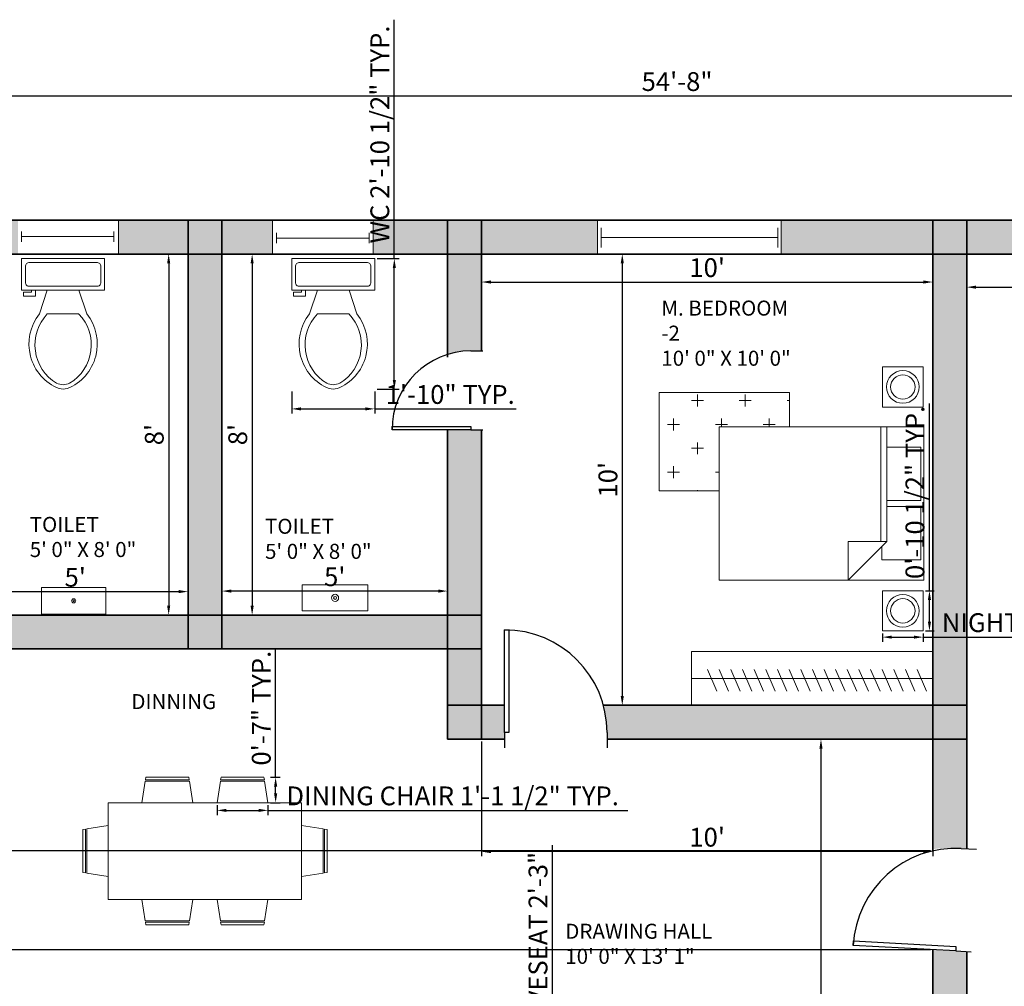
# Model space of a CAD drawing. Units: millimetres. Extents: x 2768 to 4359, y 795 to 1583.
# Tile 4 of 13: x 2965 to 3226, y 1286 to 1543. Entities that reach past the tile are written whole.
import ezdxf

# ---------------------------------------------------------------- set-up
doc = ezdxf.new("R2010")
doc.units = ezdxf.units.MM
for name, color, linetype, lineweight in [('A-ANNO-DIMS', 90, 'Continuous', 18), ('A-AREA-IDEN', 190, 'Continuous', 18), ('A-FLOR-CASE', 50, 'Continuous', 18), ('A-FLOR-CASE-PATT', 50, 'Continuous', 13), ('A-FLOR-FIXT', 50, 'Continuous', 18), ('A-FURN-PATT', 50, 'Continuous', 9), ('A-WALL-PATT', 140, 'Continuous', 9), ('doors', 10, 'Continuous', 25), ('furniture', 50, 'Continuous', 18), ('walls', 140, 'Continuous', 35), ('windows', 30, 'Continuous', 18)]:
    doc.layers.add(name, color=color, linetype=linetype, lineweight=lineweight)
doc.styles.get("Standard").update_dxf_attribs({"font": 'arial.ttf'})
doc.dimstyles.new('ISO-25', dxfattribs={"dimtxt": 5, "dimasz": 2.5, "dimexe": 1.25, "dimexo": 0.625, "dimtad": 1, "dimdec": 0, "dimlunit": 3, "dimtxsty": 'Standard', "dimcen": 2.5, "dimadec": 0, "dimazin": 0, "dimtfac": 1, "dimtdec": 0, "dimtmove": 0, "dimatfit": 3, "dimfxl": 1, "dimarcsym": 0})

# ---------------------------------------------------------------- blocks, each defined once
blk = doc.blocks.new('*U2')
for p, q in [((0, 0), (0, -6)), ((40, 0), (40, -6))]:
    blk.add_line(p, q)
blk.add_lwpolyline([(0, 0), (0, 40), (1.75, 40), (1.75, 0)], close=True)
blk.add_arc((0, 0), 40, 0, 90)
blk = doc.blocks.new('*U4')
for p, q in [((0, 4), (0, 0)), ((36, 4), (36, 0)), ((0, 2), (36, 2))]:
    blk.add_line(p, q)
blk = doc.blocks.new('*U5')
for p, q in [((0, 4), (0, 0)), ((36, 4), (36, 0)), ((0, 2), (36, 2))]:
    blk.add_line(p, q)
blk = doc.blocks.new('Toilet - top')
for p, q in [((9.5, -6), (9.5, -2)), ((-10, -8.5), (-8, -8.5)), ((-10, -9.5), (-10, -8.5)), ((-7, -9.5), (-10, -9.5)), ((-8, -8.5), (-8, -8)), ((-7, -8), (-7, -9.5)), ((-4, -8), (-6, -14)), ((4, -8), (6, -14)), ((4, -14), (-4, -14))]:
    blk.add_line(p, q)
blk.add_lwpolyline([(10.5, -8), (10.5, 0), (-10.5, 0), (-10.5, -8)], close=True)
for points in [[(-9.5, -2), (-9.5, -6)], [(8.5, -1), (-8.5, -1)], [(-8.5, -7), (8.5, -7)]]:
    blk.add_lwpolyline(points)
for centre, radius, start, end in [((-8.62, -1.88), 0.884, 81.8699, 188.1301), ((8.62, -1.88), 0.884, 351.8699, 98.1301), ((-8.62, -6.12), 0.884, 171.8699, 278.1301), ((8.62, -6.12), 0.884, 261.8699, 8.1301), ((3.52, -21.58), 12.17, 141.4691, 247.9714), ((4.2, -21.82), 11.33, 136.3677, 238.9468), ((-3.52, -21.58), 12.17, 292.0284, 38.5307), ((-4.2, -21.82), 11.33, 301.053, 43.6321), ((0, -27.88), 4, 245.7318, 294.2682), ((0, -29), 4, 254.8605, 285.1395)]:
    blk.add_arc(centre, radius, start, end)
blk = doc.blocks.new('*D15')
at = {"layer": 'A-ANNO-DIMS', "color": 0, "lineweight": -2, "transparency": 16777216}
for p, q in [((3003.1, 1480.41), (3005.5, 1480.41)), ((3004.25, 1477.91), (3004.25, 1386.91)), ((3003.1, 1384.41), (3005.5, 1384.41))]:
    blk.add_line(p, q, dxfattribs=at)
at = {"layer": 'A-ANNO-DIMS', "color": 0, "transparency": 16777216}
for points in [[(3003.83, 1477.91), (3004.66, 1477.91), (3004.25, 1480.41)], [(3003.83, 1386.91), (3004.66, 1386.91), (3004.25, 1384.41)]]:
    blk.add_solid(points, dxfattribs=at)
at = {"layer": 'Defpoints', "color": 0, "transparency": 16777216}
for p in [(3002.47, 1480.41), (3002.47, 1384.41), (3004.25, 1384.41)]:
    blk.add_point(p, dxfattribs=at)
at = {"layer": 'A-ANNO-DIMS', "color": 0, "transparency": 16777216, "insert": (3001.07, 1432.41), "char_height": 5, "attachment_point": 5, "rotation": 90}
blk.add_mtext("8'", dxfattribs=at)
blk = doc.blocks.new('*D16')
at = {"layer": 'A-ANNO-DIMS', "color": 0, "lineweight": -2, "transparency": 16777216}
for p, q in [((2949.41, 1391.28), (2949.41, 1391.9)), ((2951.91, 1390.65), (3006.91, 1390.65)), ((3009.41, 1391.28), (3009.41, 1391.9))]:
    blk.add_line(p, q, dxfattribs=at)
at = {"layer": 'A-ANNO-DIMS', "color": 0, "transparency": 16777216}
for points in [[(2951.91, 1391.07), (2951.91, 1390.23), (2949.41, 1390.65)], [(3006.91, 1391.07), (3006.91, 1390.23), (3009.41, 1390.65)]]:
    blk.add_solid(points, dxfattribs=at)
at = {"layer": 'Defpoints', "color": 0, "transparency": 16777216}
for p in [(2949.41, 1390.65), (3009.41, 1390.65), (3009.41, 1390.65)]:
    blk.add_point(p, dxfattribs=at)
at = {"layer": 'A-ANNO-DIMS', "color": 0, "transparency": 16777216, "insert": (2979.41, 1393.82), "char_height": 5, "attachment_point": 5}
blk.add_mtext("5'", dxfattribs=at)
blk = doc.blocks.new('*D17')
at = {"layer": 'A-ANNO-DIMS', "color": 0, "lineweight": -2, "transparency": 16777216}
for p, q in [((3024.99, 1480.41), (3027.69, 1480.41)), ((3026.44, 1477.91), (3026.44, 1386.91)), ((3024.99, 1384.41), (3027.69, 1384.41))]:
    blk.add_line(p, q, dxfattribs=at)
at = {"layer": 'A-ANNO-DIMS', "color": 0, "transparency": 16777216}
for points in [[(3026.02, 1477.91), (3026.85, 1477.91), (3026.44, 1480.41)], [(3026.02, 1386.91), (3026.85, 1386.91), (3026.44, 1384.41)]]:
    blk.add_solid(points, dxfattribs=at)
at = {"layer": 'Defpoints', "color": 0, "transparency": 16777216}
for p in [(3024.37, 1480.41), (3024.37, 1384.41), (3026.44, 1384.41)]:
    blk.add_point(p, dxfattribs=at)
at = {"layer": 'A-ANNO-DIMS', "color": 0, "transparency": 16777216, "insert": (3023.26, 1432.41), "char_height": 5, "attachment_point": 5, "rotation": 90}
blk.add_mtext("8'", dxfattribs=at)
blk = doc.blocks.new('*D18')
at = {"layer": 'A-ANNO-DIMS', "color": 0, "lineweight": -2, "transparency": 16777216}
for p, q in [((3018.41, 1390.69), (3018.41, 1392.04)), ((3075.91, 1390.79), (3020.91, 1390.79)), ((3078.41, 1390.69), (3078.41, 1392.04))]:
    blk.add_line(p, q, dxfattribs=at)
at = {"layer": 'A-ANNO-DIMS', "color": 0, "transparency": 16777216}
for points in [[(3020.91, 1391.21), (3020.91, 1390.37), (3018.41, 1390.79)], [(3075.91, 1391.21), (3075.91, 1390.37), (3078.41, 1390.79)]]:
    blk.add_solid(points, dxfattribs=at)
at = {"layer": 'Defpoints', "color": 0, "transparency": 16777216}
for p in [(3018.41, 1390.79), (3018.41, 1390.07), (3078.41, 1390.07)]:
    blk.add_point(p, dxfattribs=at)
at = {"layer": 'A-ANNO-DIMS', "color": 0, "transparency": 16777216, "insert": (3048.41, 1393.96), "char_height": 5, "attachment_point": 5}
blk.add_mtext("5'", dxfattribs=at)
blk = doc.blocks.new('*D19')
at = {"layer": 'A-ANNO-DIMS', "color": 0, "lineweight": -2, "transparency": 16777216}
for p, q in [((3087.41, 1474.21), (3087.41, 1471.72)), ((3207.41, 1474.21), (3207.41, 1471.72)), ((3089.91, 1472.97), (3204.91, 1472.97))]:
    blk.add_line(p, q, dxfattribs=at)
at = {"layer": 'A-ANNO-DIMS', "color": 0, "transparency": 16777216}
for points in [[(3089.91, 1473.39), (3089.91, 1472.56), (3087.41, 1472.97)], [(3204.91, 1473.39), (3204.91, 1472.56), (3207.41, 1472.97)]]:
    blk.add_solid(points, dxfattribs=at)
at = {"layer": 'Defpoints', "color": 0, "transparency": 16777216}
for p in [(3087.41, 1474.83), (3207.41, 1474.83), (3207.41, 1472.97)]:
    blk.add_point(p, dxfattribs=at)
at = {"layer": 'A-ANNO-DIMS', "color": 0, "transparency": 16777216, "insert": (3147.41, 1476.15), "char_height": 5, "attachment_point": 5}
blk.add_mtext("10'", dxfattribs=at)
blk = doc.blocks.new('*D20')
at = {"layer": 'A-ANNO-DIMS', "color": 0, "lineweight": -2, "transparency": 16777216}
for p, q in [((3129.29, 1480.41), (3123.59, 1480.41)), ((3124.84, 1477.91), (3124.84, 1362.91)), ((3129.29, 1360.41), (3123.59, 1360.41))]:
    blk.add_line(p, q, dxfattribs=at)
at = {"layer": 'A-ANNO-DIMS', "color": 0, "transparency": 16777216}
for points in [[(3124.43, 1477.91), (3125.26, 1477.91), (3124.84, 1480.41)], [(3124.43, 1362.91), (3125.26, 1362.91), (3124.84, 1360.41)]]:
    blk.add_solid(points, dxfattribs=at)
at = {"layer": 'Defpoints', "color": 0, "transparency": 16777216}
for p in [(3129.91, 1480.41), (3124.84, 1360.41), (3129.91, 1360.41)]:
    blk.add_point(p, dxfattribs=at)
at = {"layer": 'A-ANNO-DIMS', "color": 0, "transparency": 16777216, "insert": (3121.67, 1420.41), "char_height": 5, "attachment_point": 5, "rotation": 90}
blk.add_mtext("10'", dxfattribs=at)
blk = doc.blocks.new('*D29')
at = {"layer": 'A-ANNO-DIMS', "color": 0, "lineweight": -2, "transparency": 16777216}
for p, q in [((3087.41, 1350.78), (3087.41, 1320.27)), ((3207.41, 1350.78), (3207.41, 1320.27)), ((3204.91, 1321.52), (3089.91, 1321.52))]:
    blk.add_line(p, q, dxfattribs=at)
at = {"layer": 'A-ANNO-DIMS', "color": 0, "transparency": 16777216}
for points in [[(3089.91, 1321.94), (3089.91, 1321.1), (3087.41, 1321.52)], [(3204.91, 1321.94), (3204.91, 1321.1), (3207.41, 1321.52)]]:
    blk.add_solid(points, dxfattribs=at)
at = {"layer": 'Defpoints', "color": 0, "transparency": 16777216}
for p in [(3087.41, 1351.41), (3207.41, 1351.41), (3087.41, 1321.52)]:
    blk.add_point(p, dxfattribs=at)
at = {"layer": 'A-ANNO-DIMS', "color": 0, "transparency": 16777216, "insert": (3147.41, 1324.7), "char_height": 5, "attachment_point": 5}
blk.add_mtext("10'", dxfattribs=at)
blk = doc.blocks.new('*D30')
at = {"layer": 'A-ANNO-DIMS', "color": 0, "lineweight": -2, "transparency": 16777216}
for p, q in [((3177.44, 1351.41), (3178.91, 1351.41)), ((3177.66, 1348.91), (3177.66, 1196.91)), ((3177.44, 1194.41), (3178.91, 1194.41))]:
    blk.add_line(p, q, dxfattribs=at)
at = {"layer": 'A-ANNO-DIMS', "color": 0, "transparency": 16777216}
for points in [[(3177.25, 1348.91), (3178.08, 1348.91), (3177.66, 1351.41)], [(3177.25, 1196.91), (3178.08, 1196.91), (3177.66, 1194.41)]]:
    blk.add_solid(points, dxfattribs=at)
at = {"layer": 'Defpoints', "color": 0, "transparency": 16777216}
for p in [(3176.82, 1351.41), (3176.82, 1194.41), (3177.66, 1194.41)]:
    blk.add_point(p, dxfattribs=at)
at = {"layer": 'A-ANNO-DIMS', "color": 0, "transparency": 16777216, "insert": (3174.48, 1272.91), "char_height": 5, "attachment_point": 5, "rotation": 90}
blk.add_mtext('13\'-1"', dxfattribs=at)
blk = doc.blocks.new('*D36')
at = {"layer": 'A-ANNO-DIMS', "color": 0, "lineweight": -2, "transparency": 16777216}
for p, q in [((3216.41, 1480.21), (3216.41, 1470.35)), ((3458.41, 1480.21), (3458.41, 1470.35)), ((3218.91, 1471.6), (3455.91, 1471.6))]:
    blk.add_line(p, q, dxfattribs=at)
at = {"layer": 'A-ANNO-DIMS', "color": 0, "transparency": 16777216}
for points in [[(3218.91, 1472.02), (3218.91, 1471.19), (3216.41, 1471.6)], [(3455.91, 1472.02), (3455.91, 1471.19), (3458.41, 1471.6)]]:
    blk.add_solid(points, dxfattribs=at)
at = {"layer": 'Defpoints', "color": 0, "transparency": 16777216}
for p in [(3216.41, 1480.83), (3458.41, 1480.83), (3458.41, 1471.6)]:
    blk.add_point(p, dxfattribs=at)
at = {"layer": 'A-ANNO-DIMS', "color": 0, "transparency": 16777216, "insert": (3337.41, 1474.78), "char_height": 5, "attachment_point": 5}
blk.add_mtext('20\'-2"', dxfattribs=at)
blk = doc.blocks.new('CHAIR-DINING')
for p, q in [((0.89, 5.71), (0, 0)), ((0.9, 5.71), (12.65, 5.71)), ((1.06, 6.78), (0.95, 6.07)), ((12.59, 6.07), (0.95, 6.07)), ((1.06, 6.78), (12.48, 6.78)), ((12.59, 6.07), (12.48, 6.78)), ((13.54, 0), (12.65, 5.71))]:
    blk.add_line(p, q)
blk = doc.blocks.new('NIGHTSTAND-RECT-B')
blk.add_lwpolyline([(0, 10.72), (10.88, 10.72), (10.88, 0), (0, 0)], close=True)
for radius in [4.35, 3.24]:
    blk.add_circle((5.44, 5.36), radius)
blk = doc.blocks.new('*D77')
at = {"layer": 'A-ANNO-DIMS', "color": 0, "lineweight": -2, "transparency": 16777216}
for p, q in [((3064.24, 1479.19), (3064.24, 1542.73)), ((3059.65, 1479.19), (3065.49, 1479.19)), ((3064.24, 1446.95), (3064.24, 1476.69)), ((3059.65, 1444.45), (3065.49, 1444.45))]:
    blk.add_line(p, q, dxfattribs=at)
at = {"layer": 'A-ANNO-DIMS', "color": 0, "transparency": 16777216}
for points in [[(3063.82, 1476.69), (3064.66, 1476.69), (3064.24, 1479.19)], [(3063.82, 1446.95), (3064.66, 1446.95), (3064.24, 1444.45)]]:
    blk.add_solid(points, dxfattribs=at)
at = {"layer": 'Defpoints', "color": 0, "transparency": 16777216}
for p in [(3059.03, 1479.19), (3064.24, 1479.19), (3059.03, 1444.45)]:
    blk.add_point(p, dxfattribs=at)
at = {"layer": 'A-ANNO-DIMS', "color": 0, "transparency": 16777216, "insert": (3061.03, 1512.21), "char_height": 5, "attachment_point": 5, "rotation": 90}
blk.add_mtext('WC 2\'-10 1/2" TYP.', dxfattribs=at)
blk = doc.blocks.new('*D78')
at = {"layer": 'A-ANNO-DIMS', "color": 0, "lineweight": -2, "transparency": 16777216}
for p, q in [((3036.95, 1443.83), (3036.95, 1437.99)), ((3059.03, 1443.83), (3059.03, 1437.99)), ((3039.45, 1439.24), (3056.53, 1439.24)), ((3059.03, 1439.24), (3096.67, 1439.24))]:
    blk.add_line(p, q, dxfattribs=at)
at = {"layer": 'A-ANNO-DIMS', "color": 0, "transparency": 16777216}
for points in [[(3039.45, 1439.66), (3039.45, 1438.82), (3036.95, 1439.24)], [(3056.53, 1439.66), (3056.53, 1438.82), (3059.03, 1439.24)]]:
    blk.add_solid(points, dxfattribs=at)
at = {"layer": 'Defpoints', "color": 0, "transparency": 16777216}
for p in [(3036.95, 1444.45), (3059.03, 1444.45), (3059.03, 1439.24)]:
    blk.add_point(p, dxfattribs=at)
at = {"layer": 'A-ANNO-DIMS', "color": 0, "transparency": 16777216, "insert": (3079.1, 1442.42), "char_height": 5, "attachment_point": 5}
blk.add_mtext('1\'-10" TYP.', dxfattribs=at)
blk = doc.blocks.new('*D93')
at = {"layer": 'A-ANNO-DIMS', "color": 0, "lineweight": -2, "transparency": 16777216}
for p, q in [((3017.11, 1333.88), (3017.11, 1331.22)), ((3019.61, 1332.47), (3028.15, 1332.47)), ((3030.65, 1333.88), (3030.65, 1331.22)), ((3030.65, 1332.47), (3126.34, 1332.47))]:
    blk.add_line(p, q, dxfattribs=at)
at = {"layer": 'A-ANNO-DIMS', "color": 0, "transparency": 16777216}
for points in [[(3019.61, 1332.89), (3019.61, 1332.05), (3017.11, 1332.47)], [(3028.15, 1332.89), (3028.15, 1332.05), (3030.65, 1332.47)]]:
    blk.add_solid(points, dxfattribs=at)
at = {"layer": 'Defpoints', "color": 0, "transparency": 16777216}
for p in [(3017.11, 1334.5), (3030.65, 1334.5), (3030.65, 1332.47)]:
    blk.add_point(p, dxfattribs=at)
at = {"layer": 'A-ANNO-DIMS', "color": 0, "transparency": 16777216, "insert": (3079.75, 1335.68), "char_height": 5, "attachment_point": 5}
blk.add_mtext('DINING CHAIR 1\'-1 1/2" TYP.', dxfattribs=at)
blk = doc.blocks.new('*D94')
at = {"layer": 'A-ANNO-DIMS', "color": 0, "lineweight": -2, "transparency": 16777216}
for p, q in [((3032.68, 1341.28), (3032.68, 1375.51)), ((3031.28, 1341.28), (3033.93, 1341.28)), ((3032.68, 1337), (3032.68, 1338.78)), ((3031.28, 1334.5), (3033.93, 1334.5))]:
    blk.add_line(p, q, dxfattribs=at)
at = {"layer": 'A-ANNO-DIMS', "color": 0, "transparency": 16777216}
for points in [[(3032.27, 1338.78), (3033.1, 1338.78), (3032.68, 1341.28)], [(3032.27, 1337), (3033.1, 1337), (3032.68, 1334.5)]]:
    blk.add_solid(points, dxfattribs=at)
at = {"layer": 'Defpoints', "color": 0, "transparency": 16777216}
for p in [(3030.65, 1341.28), (3032.68, 1341.28), (3030.65, 1334.5)]:
    blk.add_point(p, dxfattribs=at)
at = {"layer": 'A-ANNO-DIMS', "color": 0, "transparency": 16777216, "insert": (3029.51, 1359.65), "char_height": 5, "attachment_point": 5, "rotation": 90}
blk.add_mtext('0\'-7" TYP.', dxfattribs=at)
blk = doc.blocks.new('*D109')
at = {"layer": 'A-ANNO-DIMS', "color": 0, "lineweight": -2, "transparency": 16777216}
for p, q in [((3106.3, 1267.57), (3106.3, 1323.21)), ((3102.89, 1267.57), (3107.55, 1267.57)), ((3106.3, 1243.13), (3106.3, 1265.07)), ((3102.89, 1240.63), (3107.55, 1240.63))]:
    blk.add_line(p, q, dxfattribs=at)
at = {"layer": 'A-ANNO-DIMS', "color": 0, "transparency": 16777216}
for points in [[(3105.89, 1265.07), (3106.72, 1265.07), (3106.3, 1267.57)], [(3105.89, 1243.13), (3106.72, 1243.13), (3106.3, 1240.63)]]:
    blk.add_solid(points, dxfattribs=at)
at = {"layer": 'Defpoints', "color": 0, "transparency": 16777216}
for p in [(3102.26, 1267.57), (3106.3, 1267.57), (3102.26, 1240.63)]:
    blk.add_point(p, dxfattribs=at)
at = {"layer": 'A-ANNO-DIMS', "color": 0, "transparency": 16777216, "insert": (3103.09, 1296.64), "char_height": 5, "attachment_point": 5, "rotation": 90}
blk.add_mtext('LOVESEAT 2\'-3"', dxfattribs=at)
blk = doc.blocks.new('*D119')
at = {"layer": 'A-ANNO-DIMS', "color": 0, "lineweight": -2, "transparency": 16777216}
for p, q in [((3193.99, 1379.55), (3193.99, 1377.29)), ((3204.87, 1379.55), (3204.87, 1377.29)), ((3196.49, 1378.54), (3202.37, 1378.54)), ((3204.87, 1378.54), (3296.68, 1378.54))]:
    blk.add_line(p, q, dxfattribs=at)
at = {"layer": 'A-ANNO-DIMS', "color": 0, "transparency": 16777216}
for points in [[(3196.49, 1378.96), (3196.49, 1378.13), (3193.99, 1378.54)], [(3202.37, 1378.96), (3202.37, 1378.13), (3204.87, 1378.54)]]:
    blk.add_solid(points, dxfattribs=at)
at = {"layer": 'Defpoints', "color": 0, "transparency": 16777216}
for p in [(3193.99, 1380.18), (3204.87, 1380.18), (3204.87, 1378.54)]:
    blk.add_point(p, dxfattribs=at)
at = {"layer": 'A-ANNO-DIMS', "color": 0, "transparency": 16777216, "insert": (3252.03, 1381.75), "char_height": 5, "attachment_point": 5}
blk.add_mtext('NIGHTSTAND B 0\'-11" TYP.', dxfattribs=at)
blk = doc.blocks.new('*D120')
at = {"layer": 'A-ANNO-DIMS', "color": 0, "lineweight": -2, "transparency": 16777216}
for p, q in [((3206.5, 1390.9), (3206.5, 1440.66)), ((3205.5, 1390.9), (3207.75, 1390.9)), ((3206.5, 1382.68), (3206.5, 1388.4)), ((3205.5, 1380.18), (3207.75, 1380.18))]:
    blk.add_line(p, q, dxfattribs=at)
at = {"layer": 'A-ANNO-DIMS', "color": 0, "transparency": 16777216}
for points in [[(3206.09, 1388.4), (3206.92, 1388.4), (3206.5, 1390.9)], [(3206.09, 1382.68), (3206.92, 1382.68), (3206.5, 1380.18)]]:
    blk.add_solid(points, dxfattribs=at)
at = {"layer": 'Defpoints', "color": 0, "transparency": 16777216}
for p in [(3204.87, 1390.9), (3206.5, 1390.9), (3204.87, 1380.18)]:
    blk.add_point(p, dxfattribs=at)
at = {"layer": 'A-ANNO-DIMS', "color": 0, "transparency": 16777216, "insert": (3203.29, 1417.03), "char_height": 5, "attachment_point": 5, "rotation": 90}
blk.add_mtext('0\'-10 1/2" TYP.', dxfattribs=at)
blk = doc.blocks.new('*D125')
at = {"layer": 'A-ANNO-DIMS', "color": 0, "lineweight": -2, "transparency": 16777216}
for p, q in [((2811.41, 1490.03), (2811.41, 1523.71)), ((3467.41, 1490.03), (3467.41, 1523.71)), ((2813.91, 1522.46), (3464.91, 1522.46))]:
    blk.add_line(p, q, dxfattribs=at)
at = {"layer": 'A-ANNO-DIMS', "color": 0, "transparency": 16777216}
for points in [[(2813.91, 1522.87), (2813.91, 1522.04), (2811.41, 1522.46)], [(3464.91, 1522.87), (3464.91, 1522.04), (3467.41, 1522.46)]]:
    blk.add_solid(points, dxfattribs=at)
at = {"layer": 'Defpoints', "color": 0, "transparency": 16777216}
for p in [(3467.41, 1522.46), (2811.41, 1489.41), (3467.41, 1489.41)]:
    blk.add_point(p, dxfattribs=at)
at = {"layer": 'A-ANNO-DIMS', "color": 0, "transparency": 16777216, "insert": (3139.41, 1525.63), "char_height": 5, "attachment_point": 5}
blk.add_mtext('54\'-8"', dxfattribs=at)
blk = doc.blocks.new('*D131')
at = {"layer": 'A-ANNO-DIMS', "color": 0, "lineweight": -2, "transparency": 16777216}
for p, q in [((3206.78, 1321.72), (2777.11, 1321.72)), ((2778.36, 1297.93), (2778.36, 1319.22)), ((3206.78, 1295.43), (2777.11, 1295.43))]:
    blk.add_line(p, q, dxfattribs=at)
at = {"layer": 'A-ANNO-DIMS', "color": 0, "transparency": 16777216}
for points in [[(2777.94, 1319.22), (2778.77, 1319.22), (2778.36, 1321.72)], [(2777.94, 1297.93), (2778.77, 1297.93), (2778.36, 1295.43)]]:
    blk.add_solid(points, dxfattribs=at)
at = {"layer": 'Defpoints', "color": 0, "transparency": 16777216}
for p in [(2778.36, 1321.72), (3207.41, 1321.72), (3207.41, 1295.43)]:
    blk.add_point(p, dxfattribs=at)
at = {"layer": 'A-ANNO-DIMS', "color": 0, "transparency": 16777216, "insert": (2775.15, 1308.58), "char_height": 5, "attachment_point": 5, "rotation": 90}
blk.add_mtext('2\'-2 1/2"', dxfattribs=at)

msp = doc.modelspace()

# ---------------------------------------------------------------- hatches: boundary and pattern name
at = {"layer": 'A-FLOR-CASE-PATT'}
h = msp.add_hatch(dxfattribs=at)
h.set_pattern_fill('ANSI31', color=256, scale=0.894999, angle=68.514, style=0)
h.paths.add_polyline_path([(3203.48, 1369.91), (3205.98, 1364.18), (3147.1, 1364.18), (3144.6, 1369.91)])
at = {"layer": 'A-FURN-PATT'}
h = msp.add_hatch(dxfattribs=at)
h.set_pattern_fill('CROSS', color=256)
h.paths.add_polyline_path([(3150.58, 1434.48), (3169.28, 1434.48), (3169.28, 1443.62), (3134.64, 1443.62), (3134.64, 1417.47), (3150.58, 1417.47)])
at = {"layer": 'A-WALL-PATT'}
h = msp.add_hatch(color=256, dxfattribs=at)
h.dxf.hatch_style = 1
h.paths.add_polyline_path([(2820.41, 1480.41), (2811.41, 1480.41), (2811.41, 1360.41), (2820.41, 1360.41)])
h.paths.add_polyline_path([(2820.41, 1489.41), (2811.41, 1489.41), (2811.41, 1480.41), (2820.41, 1480.41)])
h.paths.add_polyline_path([(2845.83, 1489.41), (2820.41, 1489.41), (2820.41, 1480.41), (2845.83, 1480.41)])
h.paths.add_polyline_path([(2940.41, 1489.41), (2894.95, 1489.41), (2894.95, 1480.41), (2940.41, 1480.41)])
h.paths.add_polyline_path([(2949.41, 1489.41), (2940.41, 1489.41), (2940.41, 1480.41), (2949.41, 1480.41)])
h.paths.add_polyline_path([(2949.41, 1480.41), (2940.41, 1480.41), (2940.41, 1433.68), (2943.15, 1433.68), (2949.41, 1433.68)])
h.paths.add_polyline_path([(2964.2, 1489.41), (2949.41, 1489.41), (2949.41, 1480.41), (2964.2, 1480.41)])
h.paths.add_polyline_path([(3018.41, 1489.41), (3009.41, 1489.41), (3009.41, 1480.41), (3018.41, 1480.41)])
h.paths.add_polyline_path([(3009.41, 1489.41), (2990.92, 1489.41), (2990.92, 1480.41), (3009.41, 1480.41)])
h.paths.add_polyline_path([(3018.41, 1480.41), (3009.41, 1480.41), (3009.41, 1384.41), (3018.41, 1384.41)])
h.paths.add_polyline_path([(3009.41, 1384.41), (2949.41, 1384.41), (2949.41, 1375.41), (3009.41, 1375.41)])
h.paths.add_polyline_path([(3018.41, 1384.41), (3009.41, 1384.41), (3009.41, 1375.41), (3018.41, 1375.41)])
h.paths.add_polyline_path([(2949.41, 1384.41), (2940.41, 1384.41), (2940.41, 1375.41), (2949.41, 1375.41)])
h.paths.add_polyline_path([(2949.41, 1413.64, -0.075856), (2943.15, 1412.69), (2940.41, 1412.69), (2940.41, 1384.41), (2949.41, 1384.41)])
h.paths.add_polyline_path([(2949.41, 1375.41), (2940.41, 1375.41), (2940.41, 1360.41), (2949.41, 1360.41)])
h.paths.add_polyline_path([(2949.41, 1360.41), (2940.41, 1360.41), (2940.41, 1351.41), (2949.41, 1351.41)])
h.paths.add_polyline_path([(2940.41, 1360.41), (2929.82, 1360.41, -0.054277), (2930.46, 1354.53), (2930.46, 1351.41), (2940.41, 1351.41)])
h.paths.add_polyline_path([(2903.16, 1354.53), (2903.16, 1360.41), (2895.41, 1360.41), (2895.41, 1351.41), (2903.16, 1351.41)])
h.paths.add_polyline_path([(2886.41, 1360.41), (2820.41, 1360.41), (2820.41, 1351.41), (2886.41, 1351.41)])
h.paths.add_polyline_path([(2895.41, 1360.41), (2886.41, 1360.41), (2886.41, 1351.41), (2895.41, 1351.41)])
h.paths.add_polyline_path([(2820.41, 1360.41), (2811.41, 1360.41), (2811.41, 1351.41), (2820.41, 1351.41)])
h.paths.add_polyline_path([(2820.41, 1351.41), (2811.41, 1351.41), (2811.41, 1213.41), (2820.41, 1213.41)])
h.paths.add_polyline_path([(2886.41, 1213.41), (2820.41, 1213.41), (2820.41, 1204.41), (2886.41, 1204.41)])
h.paths.add_polyline_path([(2820.41, 1213.41), (2811.41, 1213.41), (2811.41, 1204.41), (2820.41, 1204.41)])
h.paths.add_polyline_path([(2895.41, 1302), (2886.41, 1302), (2886.41, 1264.47), (2895.41, 1264.47)])
h.paths.add_polyline_path([(2934.05, 1209.82), (2934.05, 1213.41), (2895.41, 1213.41), (2895.41, 1204.41), (2934.59, 1204.41, -0.049949)])
h.paths.add_polyline_path([(2895.41, 1213.41), (2886.41, 1213.41), (2886.41, 1204.41), (2895.41, 1204.41)])
h.paths.add_polyline_path([(3078.41, 1384.41), (3018.41, 1384.41), (3018.41, 1375.41), (3078.41, 1375.41)])
h.paths.add_polyline_path([(3087.41, 1433.68), (3084.62, 1433.68), (3078.41, 1433.68), (3078.41, 1384.41), (3087.41, 1384.41)])
h.paths.add_polyline_path([(3087.41, 1384.41), (3078.41, 1384.41), (3078.41, 1375.41), (3087.41, 1375.41)])
h.paths.add_polyline_path([(3087.41, 1375.41), (3078.41, 1375.41), (3078.41, 1360.41), (3087.41, 1360.41)])
h.paths.add_polyline_path([(3087.41, 1360.41), (3078.41, 1360.41), (3078.41, 1351.41), (3087.41, 1351.41)])
h.paths.add_polyline_path([(3093.5, 1360.41), (3087.41, 1360.41), (3087.41, 1351.41), (3093.5, 1351.41), (3093.5, 1353.18)])
h.paths.add_polyline_path([(3207.41, 1360.41), (3119.82, 1360.41, -0.067042), (3120.8, 1353.18), (3120.8, 1351.41), (3207.41, 1351.41)])
h.paths.add_polyline_path([(3216.41, 1480.41), (3207.41, 1480.41), (3207.41, 1360.41), (3216.41, 1360.41)])
h.paths.add_polyline_path([(3216.41, 1360.41), (3207.41, 1360.41), (3207.41, 1351.41), (3216.41, 1351.41)])
h.paths.add_polyline_path([(3216.41, 1489.41), (3207.41, 1489.41), (3207.41, 1480.41), (3216.41, 1480.41)])
h.paths.add_polyline_path([(3207.41, 1489.41), (3167.11, 1489.41), (3167.11, 1480.41), (3207.41, 1480.41)])
h.paths.add_polyline_path([(3118.27, 1489.41), (3087.41, 1489.41), (3087.41, 1480.41), (3118.27, 1480.41)])
h.paths.add_polyline_path([(3087.41, 1489.41), (3078.41, 1489.41), (3078.41, 1480.41), (3087.41, 1480.41)])
h.paths.add_polyline_path([(3087.41, 1480.41), (3078.41, 1480.41), (3078.41, 1453.72, -0.07525), (3084.62, 1454.66), (3087.41, 1454.66)])
h.paths.add_polyline_path([(3078.41, 1489.41), (3058.65, 1489.41), (3058.65, 1480.41), (3078.41, 1480.41)])
h.paths.add_polyline_path([(3031.86, 1489.41), (3018.41, 1489.41), (3018.41, 1480.41), (3031.86, 1480.41)])
h.paths.add_polyline_path([(3458.41, 1489.41), (3216.41, 1489.41), (3216.41, 1480.41), (3458.41, 1480.41)])
h.paths.add_polyline_path([(3467.41, 1489.41), (3458.41, 1489.41), (3458.41, 1480.41), (3467.41, 1480.41)])
h.paths.add_polyline_path([(3467.41, 1480.41), (3458.41, 1480.41), (3458.41, 1020.41), (3467.41, 1020.41)])
h.paths.add_polyline_path([(3458.41, 1020.41), (3216.41, 1020.41), (3216.41, 1011.41), (3458.41, 1011.41)])
h.paths.add_polyline_path([(3467.41, 1020.41), (3458.41, 1020.41), (3458.41, 1011.41), (3467.41, 1011.41)])
h.paths.add_polyline_path([(3216.41, 1080.41), (3207.41, 1080.41), (3207.41, 1020.41), (3216.41, 1020.41)])
h.paths.add_polyline_path([(3216.41, 1020.41), (3207.41, 1020.41), (3207.41, 1011.41), (3216.41, 1011.41)])
h.paths.add_polyline_path([(3207.41, 1020.41), (3151.59, 1020.41), (3151.59, 1011.41), (3207.41, 1011.41)])
h.paths.add_polyline_path([(3216.41, 1185.41), (3207.41, 1185.41), (3207.41, 1089.41), (3216.41, 1089.41)])
h.paths.add_polyline_path([(3216.41, 1089.41), (3207.41, 1089.41), (3207.41, 1080.41), (3216.41, 1080.41)])
h.paths.add_polyline_path([(3207.41, 1089.41), (3097.07, 1089.41), (3097.07, 1087.42), (3097.07, 1080.41), (3207.41, 1080.41)])
h.paths.add_polyline_path([(3216.41, 1194.41), (3207.41, 1194.41), (3207.41, 1185.41), (3216.41, 1185.41)])
h.paths.add_polyline_path([(3207.41, 1194.41), (3055.41, 1194.41), (3055.41, 1185.41), (3207.41, 1185.41)])
h.paths.add_polyline_path([(3055.41, 1194.41), (3046.41, 1194.41), (3046.41, 1185.41), (3055.41, 1185.41)])
h.paths.add_polyline_path([(3055.41, 1128.41), (3046.41, 1128.41), (3046.41, 1020.41), (3055.41, 1020.41)])
h.paths.add_polyline_path([(3055.41, 1020.41), (3046.41, 1020.41), (3046.41, 1011.41), (3055.41, 1011.41)])
h.paths.add_polyline_path([(3102.66, 1020.41), (3055.41, 1020.41), (3055.41, 1011.41), (3102.66, 1011.41)])
h.paths.add_polyline_path([(3055.41, 1137.41), (3046.41, 1137.41), (3046.41, 1128.41), (3055.41, 1128.41)])
h.paths.add_polyline_path([(3046.41, 1137.41), (2986.41, 1137.41), (2986.41, 1128.41), (3046.41, 1128.41)])
h.paths.add_polyline_path([(2986.41, 1204.41), (2977.41, 1204.41), (2977.41, 1137.41), (2986.41, 1137.41)])
h.paths.add_polyline_path([(2986.41, 1213.41), (2977.41, 1213.41), (2977.41, 1204.41), (2986.41, 1204.41)])
h.paths.add_polyline_path([(2977.41, 1213.41), (2961.35, 1213.41), (2961.35, 1209.82), (2961.35, 1204.41), (2977.41, 1204.41)])
h.paths.add_polyline_path([(2986.41, 1137.41), (2977.41, 1137.41), (2977.41, 1128.41), (2986.41, 1128.41)])
h.paths.add_polyline_path([(2986.41, 1128.41), (2977.41, 1128.41), (2977.41, 1073.04), (2980.14, 1073.04), (2986.41, 1073.04)])
h.paths.add_polyline_path([(2986.41, 1053, -0.075909), (2980.14, 1052.05), (2977.41, 1052.05), (2977.41, 1020.41), (2986.41, 1020.41)])
h.paths.add_polyline_path([(2986.41, 1020.41), (2977.41, 1020.41), (2977.41, 1011.41), (2986.41, 1011.41)])
h.paths.add_polyline_path([(2977.41, 1020.41), (2903.99, 1020.41), (2903.99, 1011.41), (2977.41, 1011.41)])
h.paths.add_polyline_path([(2820.41, 1111.04), (2811.41, 1111.04), (2811.41, 1020.41), (2820.41, 1020.41)])
h.paths.add_polyline_path([(2820.41, 1020.41), (2811.41, 1020.41), (2811.41, 1011.41), (2820.41, 1011.41)])
h.paths.add_polyline_path([(2855.32, 1020.41), (2820.41, 1020.41), (2820.41, 1011.41), (2855.32, 1011.41)])
h.paths.add_polyline_path([(2820.41, 1204.41), (2811.41, 1204.41), (2811.41, 1161.45), (2820.41, 1161.45)])
edge = h.paths.add_edge_path()
edge.add_arc((3211.84, 1295.2), 27.3, 86.9636, 99.352)
edge.add_line((3207.41, 1322.13), (3207.41, 1351.41))
edge.add_line((3207.41, 1351.41), (3216.41, 1351.41))
edge.add_line((3216.41, 1351.41), (3216.41, 1322.29))
edge.add_line((3216.41, 1322.29), (3213.29, 1322.46))
h = msp.add_hatch(color=256, dxfattribs=at)
h.dxf.hatch_style = 1
h.paths.add_polyline_path([(3216.41, 1294.96), (3213.5, 1295.11), (3207.41, 1295.43), (3207.41, 1194.41), (3216.41, 1194.41)])
h.paths.add_polyline_path([(3216.41, 1011.41), (3207.41, 1011.41), (3207.41, 891.09), (3216.41, 891.09)])
h.paths.add_polyline_path([(3467.41, 1011.41), (3458.41, 1011.41), (3458.41, 891.09), (3467.41, 891.09)])

# ---------------------------------------------------------------- linework, layer by layer
at = {"layer": 'A-FLOR-CASE'}
msp.add_line((3143.22, 1367.55), (3207.41, 1367.55), dxfattribs=at)
msp.add_lwpolyline([(3207.41, 1360.41), (3143.22, 1360.41), (3143.22, 1374.69), (3207.41, 1374.69)], close=True, dxfattribs=at)
at = {"layer": 'A-FLOR-FIXT'}
for points in [[(2970.46, 1391.72), (2987.52, 1391.72), (2987.52, 1384.68), (2970.46, 1384.68)], [(3039.75, 1385.5), (3057.24, 1385.5), (3057.24, 1392.48), (3039.75, 1392.48)]]:
    msp.add_lwpolyline(points, close=True, dxfattribs=at)
for centre, radius in [((2978.99, 1388.2), 0.537), ((2978.99, 1388.2), 0.204), ((3048.5, 1388.99), 0.936), ((3048.5, 1388.99), 0.4)]:
    msp.add_circle(centre, radius, dxfattribs=at)
at = {"layer": 'furniture'}
for p, q in [((3134.64, 1417.47), (3134.64, 1443.62)), ((3134.64, 1443.62), (3169.28, 1443.62)), ((3169.28, 1443.62), (3169.28, 1434.48)), ((3150.58, 1393.67), (3150.58, 1434.48)), ((3150.58, 1434.48), (3204.99, 1434.48)), ((3193.57, 1404.01), (3193.57, 1434.48)), ((3195.2, 1434.48), (3195.2, 1404.01)), ((3204.99, 1434.48), (3204.99, 1393.67)), ((3195.2, 1429.04), (3204.18, 1429.04)), ((3204.18, 1429.04), (3204.18, 1414.89)), ((3150.58, 1417.47), (3134.64, 1417.47)), ((3204.18, 1414.89), (3195.2, 1414.89)), ((3195.2, 1413.26), (3204.18, 1413.26)), ((3204.18, 1413.26), (3204.18, 1399.11)), ((3184.86, 1393.67), (3195.2, 1404.01)), ((3184.86, 1404.01), (3184.86, 1393.67)), ((3195.2, 1404.01), (3184.86, 1404.01)), ((3193.84, 1399.11), (3193.84, 1402.65)), ((3204.18, 1399.11), (3193.84, 1399.11)), ((3204.99, 1393.67), (3150.58, 1393.67)), ((3039.59, 1334.5), (2988.2, 1334.5)), ((2988.2, 1334.5), (2988.2, 1308.81)), ((3039.59, 1308.81), (3039.59, 1334.5)), ((2988.2, 1308.81), (3039.59, 1308.81))]:
    msp.add_line(p, q, dxfattribs=at)
at = {"layer": 'walls'}
for p, q in [((2811.41, 1489.41), (3467.41, 1489.41)), ((3009.41, 1489.41), (3009.41, 1375.41)), ((3018.41, 1489.41), (3018.41, 1375.41)), ((3078.41, 1489.41), (3078.41, 1453.01)), ((3087.41, 1489.41), (3087.41, 1454.66)), ((3207.41, 1489.41), (3207.41, 1321.72)), ((3216.41, 1489.41), (3216.41, 1322.29)), ((2811.41, 1480.41), (3467.41, 1480.41)), ((3078.41, 1433.68), (3078.41, 1351.41)), ((3087.41, 1433.68), (3087.41, 1351.41)), ((2940.41, 1384.41), (3018.41, 1384.41)), ((2940.41, 1384.41), (3087.41, 1384.41)), ((2940.41, 1375.41), (3018.41, 1375.41)), ((2940.41, 1375.41), (3087.41, 1375.41)), ((3078.41, 1360.41), (3093.5, 1360.41)), ((3119.82, 1360.41), (3216.41, 1360.41)), ((3078.41, 1351.41), (3093.5, 1351.41)), ((3120.8, 1351.41), (3216.41, 1351.41)), ((3207.41, 1295.43), (3207.41, 891.09)), ((3216.41, 1294.96), (3216.41, 891.09))]:
    msp.add_line(p, q, dxfattribs=at)
at = {"layer": 'windows'}
for p, q in [((2990.92, 1489.41), (2990.92, 1480.41)), ((3031.86, 1489.41), (3031.86, 1480.41)), ((3058.65, 1489.41), (3058.65, 1480.41)), ((3118.27, 1489.41), (3118.27, 1480.41)), ((3167.11, 1489.41), (3167.11, 1480.41))]:
    msp.add_line(p, q, dxfattribs=at)

# ---------------------------------------------------------------- block references
at = {"layer": 'A-FLOR-FIXT', "xscale": 1.051204257850905, "yscale": 1.051204257850905, "zscale": 1.051204257850905}
for p in [(2976.19, 1479.19), (3047.99, 1479.19)]:
    msp.add_blockref('Toilet - top', p, dxfattribs=at)
at = {"layer": 'doors'}
for p, xscale, yscale, zscale, rotation in [((3084.62, 1433.68), 0.5246855638968122, 0.5246855638968122, 0.5246855638968122, 89.99999999999999), ((3213.5, 1295.11), 0.6824775533392957, 0.6824775533392957, 0.6824775533392957, 86.96356957235994)]:
    msp.add_blockref('*U2', p, dxfattribs=dict(at, xscale=xscale, yscale=yscale, zscale=zscale, rotation=rotation))
at = {"layer": 'doors', "xscale": 0.6824775533392957, "yscale": 0.6824775533392957, "zscale": 0.6824775533392957}
msp.add_blockref('*U2', (3093.5, 1353.18), dxfattribs=at)
at = {"layer": 'furniture'}
for name, p in [('NIGHTSTAND-RECT-B', (3193.99, 1439.71)), ('NIGHTSTAND-RECT-B', (3193.99, 1380.18)), ('CHAIR-DINING', (2997.13, 1334.5)), ('CHAIR-DINING', (3017.11, 1334.5))]:
    msp.add_blockref(name, p, dxfattribs=at)
for p, rotation in [((2988.2, 1314.88), 90.00584970642272), ((3039.58, 1328.43), 269.9999986166262), ((3010.67, 1308.81), 180.0056718243519), ((3030.65, 1308.81), 180.0056718243519)]:
    msp.add_blockref('CHAIR-DINING', p, dxfattribs=dict(at, rotation=rotation))
at = {"layer": 'windows'}
for name, p, xscale, yscale, zscale in [('*U4', (3119.22, 1482.17), 1.304585616368386, 1.304585616368386, 1.304585616368386), ('*U5', (2965.08, 1483.67), 0.6837569988572593, 0.6837569988572593, 0.6837569988572593), ('*U5', (3032.94, 1483.28), 0.6837569988572593, 0.6837569988572593, 0.6837569988572593)]:
    msp.add_blockref(name, p, dxfattribs=dict(at, xscale=xscale, yscale=yscale, zscale=zscale))

# ---------------------------------------------------------------- texts
at = {"layer": 'A-AREA-IDEN', "char_height": 4, "attachment_point": 1}
for s, width, insert in [('M. BEDROOM -2 \\P10\' 0" X 10\' 0"', 35.1504, (3135.23, 1468.04)), ('TOILET\\P5\' 0" X 8\' 0"', 28.7994, (2967.31, 1410.51)), ('TOILET \\P5\' 0" X 8\' 0"', 32.1276, (3029.87, 1410.02)), ('DINNING ', 42.8523, (2994.33, 1363.4)), ('DRAWING HALL \\P10\' 0" X 13\' 1"', 48.3921, (3109.69, 1302.33))]:
    msp.add_mtext_dynamic_manual_height_columns(s, width=width, gutter_width=12.5, heights=[0], dxfattribs=dict(at, insert=insert))

# ---------------------------------------------------------------- dimensions: what is measured, and where the dimension line sits
at = {"layer": 'A-ANNO-DIMS'}
for base, p1, p2, text, picture, middle in [((3064.24, 1479.19), (3059.03, 1444.45), (3059.03, 1479.19), 'WC <> TYP.', '*D77', (3061.03, 1512.21)), ((3206.5, 1390.9), (3204.87, 1380.18), (3204.87, 1390.9), '<> TYP.', '*D120', (3203.29, 1417.03)), ((3032.68, 1341.28), (3030.65, 1334.5), (3030.65, 1341.28), '<> TYP.', '*D94', (3029.51, 1359.65)), ((3106.3, 1267.57), (3102.26, 1240.63), (3102.26, 1267.57), 'LOVESEAT <>', '*D109', (3103.09, 1296.64))]:
    dim = msp.add_linear_dim(base=base, p1=p1, p2=p2, angle=90, text=text, dimstyle='ISO-25', override={"dimdec": 1, "dimlfac": 1, "dimrnd": 0, "dimzin": 1, "dimdsep": 46, "dimlunit": 4, "dimfrac": 2}, dxfattribs=at)
    dim.commit()
    dim.dimension.update_dxf_attribs({"geometry": picture, "text_midpoint": middle})
for base, p1, p2, override, picture, middle in [((3467.41, 1522.46), (2811.41, 1489.41), (3467.41, 1489.41), {"dimdec": 1, "dimlfac": 1, "dimrnd": 0, "dimzin": 1, "dimdsep": 46, "dimlunit": 4, "dimfrac": 2}, '*D125', (3139.41, 1525.63)), ((3207.41, 1472.97), (3087.41, 1474.83), (3207.41, 1474.83), {"dimclrd": 0, "dimclre": 0, "dimclrt": 0}, '*D19', (3147.41, 1476.15)), ((3458.41, 1471.6), (3216.41, 1480.83), (3458.41, 1480.83), {"dimclrd": 0, "dimclre": 0, "dimclrt": 0}, '*D36', (3337.41, 1474.78)), ((3009.41, 1390.65), (2949.41, 1390.65), (3009.41, 1390.65), {"dimclrd": 0, "dimclre": 0, "dimclrt": 0}, '*D16', (2979.41, 1393.82)), ((3018.41, 1390.79), (3078.41, 1390.07), (3018.41, 1390.07), {"dimclrd": 0, "dimclre": 0, "dimclrt": 0}, '*D18', (3048.41, 1393.96)), ((3087.41, 1321.52), (3207.41, 1351.41), (3087.41, 1351.41), {"dimclrd": 0, "dimclre": 0, "dimclrt": 0}, '*D29', (3147.41, 1324.7))]:
    dim = msp.add_linear_dim(base=base, p1=p1, p2=p2, dimstyle='ISO-25', override=override, dxfattribs=at)
    dim.commit()
    dim.dimension.update_dxf_attribs({"geometry": picture, "text_midpoint": middle})
for base, p1, p2, override, picture, middle in [((3004.25, 1384.41), (3002.47, 1480.41), (3002.47, 1384.41), {"dimclrd": 0, "dimclre": 0, "dimclrt": 0}, '*D15', (3001.07, 1432.41)), ((3026.44, 1384.41), (3024.37, 1480.41), (3024.37, 1384.41), {"dimclrd": 0, "dimclre": 0, "dimclrt": 0}, '*D17', (3023.26, 1432.41)), ((3124.84, 1360.41), (3129.91, 1480.41), (3129.91, 1360.41), {"dimclrd": 0, "dimclre": 0, "dimclrt": 0}, '*D20', (3121.67, 1420.41)), ((3177.66, 1194.41), (3176.82, 1351.41), (3176.82, 1194.41), {"dimclrd": 0, "dimclre": 0, "dimclrt": 0}, '*D30', (3174.48, 1272.91)), ((2778.36, 1321.72), (3207.41, 1295.43), (3207.41, 1321.72), {"dimdec": 1, "dimlfac": 1, "dimrnd": 0, "dimzin": 1, "dimdsep": 46, "dimlunit": 4, "dimfrac": 2}, '*D131', (2775.15, 1308.58))]:
    dim = msp.add_linear_dim(base=base, p1=p1, p2=p2, angle=90, dimstyle='ISO-25', override=override, dxfattribs=at)
    dim.commit()
    dim.dimension.update_dxf_attribs({"geometry": picture, "text_midpoint": middle})
for base, p1, p2, text, picture, middle in [((3059.03, 1439.24), (3036.95, 1444.45), (3059.03, 1444.45), '<> TYP.', '*D78', (3079.1, 1442.42)), ((3204.87, 1378.54), (3193.99, 1380.18), (3204.87, 1380.18), 'NIGHTSTAND B <> TYP.', '*D119', (3252.03, 1381.75)), ((3030.65, 1332.47), (3017.11, 1334.5), (3030.65, 1334.5), 'DINING CHAIR <> TYP.', '*D93', (3079.75, 1335.68))]:
    dim = msp.add_linear_dim(base=base, p1=p1, p2=p2, text=text, dimstyle='ISO-25', override={"dimdec": 1, "dimlfac": 1, "dimrnd": 0, "dimzin": 1, "dimdsep": 46, "dimlunit": 4, "dimfrac": 2}, dxfattribs=at)
    dim.commit()
    dim.dimension.update_dxf_attribs({"geometry": picture, "text_midpoint": middle})

doc.saveas('drawing.dxf')
